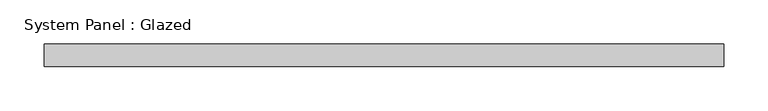
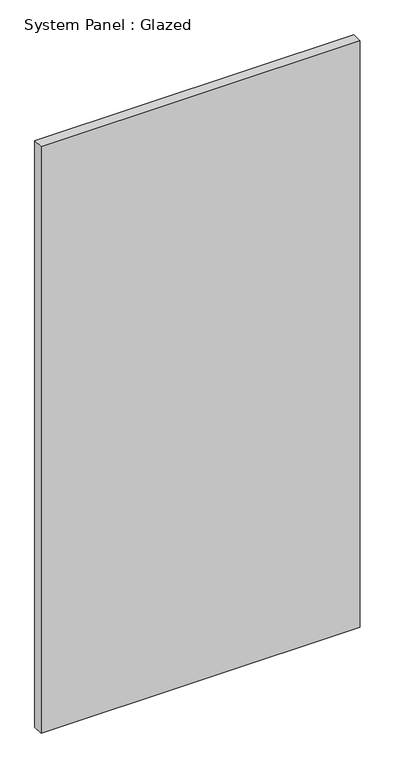
"""IFC4 building model written with IfcOpenShell, lengths in millimetres: plate geometry, System Panel : Glazed."""

from ifc_helpers import new_model, si_unit, origin, origin_with_axes, place, context, project, spatial, polyline, outline, extrude, source, transform, mapped, element, save


def system_panel_glazed_fab24249(model_context):
    return source(origin(), model_context, "Body", "SweptSolid", [
        extrude(outline(polyline([(384.175, 19.05), (-384.175, 19.05), (-384.175, 44.45), (384.175, 44.45), (384.175, 19.05)])), origin_with_axes(), (0.0, 0.0, 1.0), 1491.023499),
    ])


if __name__ == "__main__":
    model = new_model("IFC4")
    model_context = context("Model", 3, world=origin())
    ifc_project = project(units=[si_unit("LENGTHUNIT", "METRE", prefix="MILLI")], contexts=[model_context])
    site = spatial("IfcSite", under=ifc_project)
    building = spatial("IfcBuilding", under=site)
    placement = place(None, origin())
    system_panel_glazed_shape = system_panel_glazed_fab24249(model_context)
    element("IfcPlate", 1, ObjectType="System Panel : Glazed", at=placement, inside=building, context=model_context, shape_type="MappedRepresentation", body=[
        mapped(system_panel_glazed_shape, transform((0.0, 0.0, 0.0), x_axis=(1.0, 0.0, 0.0), y_axis=(0.0, 1.0, 0.0), z_axis=(0.0, 0.0, 1.0))),
    ])
    save(model, "model.ifc")

# Revit data of these elements
# Type "System Panel : Glazed"
#   Construction Type Id = "GSP4R"
#   Analytic Construction = "1/8 in Pilkington single glazing"
#   Visual Light Transmittance = 0.9
#   Solar Heat Gain Coefficient = 0.86
#   Heat Transfer Coefficient (U) = 1.18115 BTU/(h·ft²·°F)
#   Define Thermal Properties by = 1
# Element 1 (IfcPlate, "System Panel : Glazed")
#   Materials on its faces: "Glass"
# Materials
#   "Glass": class "Glass", colour RGB 0 128 192, transparency 0.75, Description = "Soda Lime Glass", Cost = 0
